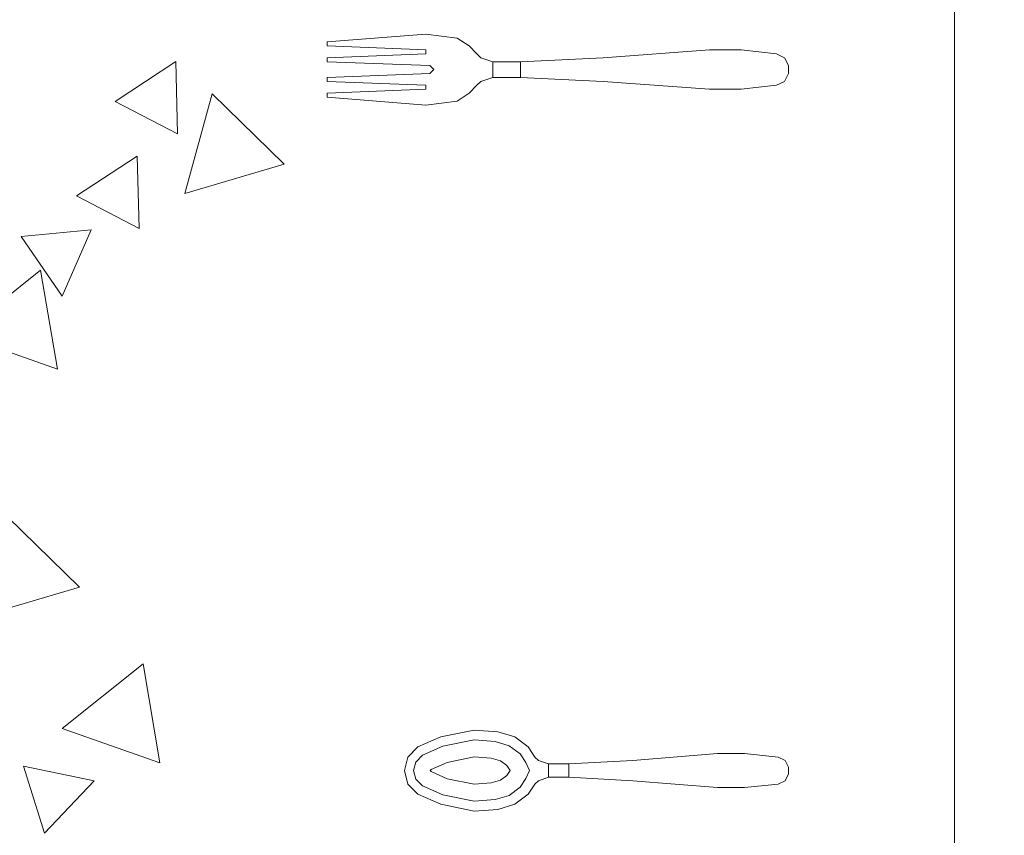
# Model space of a CAD drawing. Units: inches. Extents: x 375 to 1122, y 27 to 1069.
# Tile 37 of 155: x 731.65 to 747.02, y 283.8 to 296.54. Entities that reach past the tile are written whole.
import ezdxf

# ---------------------------------------------------------------- set-up
doc = ezdxf.new("R2010")
doc.units = ezdxf.units.IN
doc.layers.add('A-ANNO-DIMS', color=2, linetype='Continuous', lineweight=18)
doc.layers.add('Furniture', color=30, linetype='Continuous', lineweight=18)
doc.styles.get("Standard").update_dxf_attribs({"font": 'arial.ttf'})
doc.dimstyles.new('ISO-25', dxfattribs={"dimtxt": 12, "dimasz": 2.5, "dimexe": 1.5, "dimexo": 1.5, "dimtad": 1, "dimdec": 1, "dimlunit": 3, "dimtxsty": 'Standard', "dimblk": 'ARCHTICK', "dimcen": 2.5, "dimadec": 0, "dimazin": 0, "dimtfac": 1, "dimtdec": 1, "dimtmove": 0, "dimatfit": 3, "dimfxl": 1.5, "dimfxlon": 1, "dimarcsym": 0})

# ---------------------------------------------------------------- blocks, each defined once
blk = doc.blocks.new('A$C403C54AD')
for p, q in [((0.83575, 1.53256, -0.0006), (1.99923, 1.53256, -0.0006)), ((1.27568, 1.33837, -0.03581), (1.2726, 1.34298, -0.03534)), ((1.27568, 1.33837, -0.03888), (1.2726, 1.34298, -0.03842)), ((1.27287, 1.24271, -0.0006), (1.30033, 1.27073, -0.0006)), ((1.30033, 1.27073, -0.0006), (1.31179, 1.23198, -0.0006)), ((1.31179, 1.23198, -0.0006), (1.27287, 1.24271, -0.0006)), ((1.26024, 1.22842, -0.0006), (1.28849, 1.22914, -0.0006)), ((1.27579, 1.2048, -0.0006), (1.26024, 1.22842, -0.0006)), ((1.28849, 1.22914, -0.0006), (1.27579, 1.2048, -0.0006)), ((1.49552, 1.21567, -0.0006), (1.53418, 1.22227, -0.0006)), ((1.53418, 1.22227, -0.0006), (1.52076, 1.18416, -0.0006)), ((1.52076, 1.18416, -0.0006), (1.49552, 1.21567, -0.0006)), ((1.29718, 1.21338, -0.0006), (1.32543, 1.2141, -0.0006)), ((1.31273, 1.18976, -0.0006), (1.29718, 1.21338, -0.0006)), ((1.32543, 1.2141, -0.0006), (1.31273, 1.18976, -0.0006)), ((1.53546, 1.16895, -0.0006), (1.54117, 1.19665, -0.0006)), ((1.54117, 1.19665, -0.0006), (1.56166, 1.17718, -0.0006)), ((1.32856, 1.16813, -0.0006), (1.32599, 1.19547, -0.0006)), ((1.32599, 1.19547, -0.0006), (1.35188, 1.18409, -0.0006)), ((1.43807, 1.16281, -0.0006), (1.46553, 1.19082, -0.0006)), ((1.46553, 1.19082, -0.0006), (1.47699, 1.15208, -0.0006)), ((1.35188, 1.18409, -0.0006), (1.32856, 1.16813, -0.0006)), ((1.34169, 1.17565, -0.0006), (1.38035, 1.18225, -0.0006)), ((1.38035, 1.18225, -0.0006), (1.36693, 1.14415, -0.0006)), ((1.56166, 1.17718, -0.0006), (1.53546, 1.16895, -0.0006)), ((1.36693, 1.14415, -0.0006), (1.34169, 1.17565, -0.0006))]:
    blk.add_line(p, q)
for points, invisible_edges in [([(1.25875, 1.46612, -0.03397), (1.26799, 1.46612, -0.03397), (1.26953, 1.46304, -0.03421), (1.25721, 1.46304, -0.03421)], 5), ([(1.25875, 1.46612, -0.0386), (1.26799, 1.46612, -0.0386), (1.26953, 1.46304, -0.03884), (1.25721, 1.46304, -0.03884)], 5), ([(1.26491, 1.46766, -0.03413), (1.26183, 1.46766, -0.03413), (1.25875, 1.46612, -0.03397), (1.26799, 1.46612, -0.03397)], 4), ([(1.26491, 1.46766, -0.03827), (1.26183, 1.46766, -0.03827), (1.25875, 1.46612, -0.0386), (1.26799, 1.46612, -0.0386)], 4), ([(1.53323, 1.46634, -0.04237), (1.54115, 1.46634, -0.04237), (1.54247, 1.4637, -0.04257), (1.53191, 1.4637, -0.04257)], 5), ([(1.53323, 1.46634, -0.04634), (1.54115, 1.46634, -0.04634), (1.54247, 1.4637, -0.04655), (1.53191, 1.4637, -0.04655)], 5), ([(1.53851, 1.46766, -0.04251), (1.53587, 1.46766, -0.04251), (1.53323, 1.46634, -0.04237), (1.54115, 1.46634, -0.04237)], 4), ([(1.53851, 1.46766, -0.04605), (1.53587, 1.46766, -0.04605), (1.53323, 1.46634, -0.04634), (1.54115, 1.46634, -0.04634)], 4), ([(1.26953, 1.46304, -0.03421), (1.25721, 1.46304, -0.03421), (1.25567, 1.44919, -0.03425), (1.27106, 1.44919, -0.03425)], 5), ([(1.26953, 1.46304, -0.03884), (1.25721, 1.46304, -0.03884), (1.25567, 1.44919, -0.03888), (1.27106, 1.44919, -0.03888)], 5), ([(1.54247, 1.4637, -0.04257), (1.53191, 1.4637, -0.04257), (1.53059, 1.45051, -0.0426), (1.54379, 1.45051, -0.0426)], 5), ([(1.54247, 1.4637, -0.04655), (1.53191, 1.4637, -0.04655), (1.53059, 1.45051, -0.04658), (1.54379, 1.45051, -0.04658)], 5), ([(1.53059, 1.45051, -0.0426), (1.54379, 1.45051, -0.0426), (1.54379, 1.43995, -0.04232), (1.53059, 1.43995, -0.04232)], 5), ([(1.53059, 1.45051, -0.04658), (1.54379, 1.45051, -0.04658), (1.54379, 1.43995, -0.0463), (1.53059, 1.43995, -0.0463)], 5), ([(1.25567, 1.44919, -0.03425), (1.27106, 1.44919, -0.03425), (1.27106, 1.43687, -0.03392), (1.25567, 1.43687, -0.03392)], 5), ([(1.25567, 1.44919, -0.03888), (1.27106, 1.44919, -0.03888), (1.27106, 1.43687, -0.03855), (1.25567, 1.43687, -0.03855)], 5), ([(1.54379, 1.43995, -0.0463), (1.53059, 1.43995, -0.0463), (1.53323, 1.40697, -0.04292), (1.54115, 1.40697, -0.04292)], 5), ([(1.53059, 1.43995, -0.0463), (1.53059, 1.43995, -0.04232), (1.53323, 1.40697, -0.04028), (1.53323, 1.40697, -0.04292)], 4), ([(1.54379, 1.43995, -0.04232), (1.53059, 1.43995, -0.04232), (1.53323, 1.40697, -0.04028), (1.54115, 1.40697, -0.04028)], 5), ([(1.54115, 1.40697, -0.04292), (1.54115, 1.40697, -0.04028), (1.54379, 1.43995, -0.04232), (1.54379, 1.43995, -0.0463)], 1), ([(1.27106, 1.43687, -0.03392), (1.25567, 1.43687, -0.03392), (1.25875, 1.39532, -0.03153), (1.26799, 1.39532, -0.03153)], 5), ([(1.27106, 1.43687, -0.03855), (1.25567, 1.43687, -0.03855), (1.25875, 1.39532, -0.03461), (1.26799, 1.39532, -0.03461)], 5), ([(1.25567, 1.43687, -0.03855), (1.25567, 1.43687, -0.03392), (1.25875, 1.39532, -0.03153), (1.25875, 1.39532, -0.03461)], 4), ([(1.26799, 1.39532, -0.03461), (1.26799, 1.39532, -0.03153), (1.27106, 1.43687, -0.03392), (1.27106, 1.43687, -0.03855)], 1), ([(1.53323, 1.40697, -0.04028), (1.54115, 1.40697, -0.04028), (1.53983, 1.3819, -0.03779), (1.53455, 1.3819, -0.03779)], 1), ([(1.53323, 1.40697, -0.04028), (1.53323, 1.40697, -0.04292), (1.53455, 1.3819, -0.04001), (1.53455, 1.3819, -0.03779)], 5), ([(1.53323, 1.40697, -0.04292), (1.54115, 1.40697, -0.04292), (1.53983, 1.3819, -0.04001), (1.53455, 1.3819, -0.04001)], 1), ([(1.53983, 1.3819, -0.03779), (1.53983, 1.3819, -0.04001), (1.54115, 1.40697, -0.04292), (1.54115, 1.40697, -0.04028)], 5), ([(1.25875, 1.39532, -0.03153), (1.26799, 1.39532, -0.03153), (1.26645, 1.36299, -0.02863), (1.26029, 1.36299, -0.02863)], 1), ([(1.25875, 1.39532, -0.03153), (1.25875, 1.39532, -0.03461), (1.26029, 1.36299, -0.03122), (1.26029, 1.36299, -0.02863)], 5), ([(1.25875, 1.39532, -0.03461), (1.26799, 1.39532, -0.03461), (1.26645, 1.36299, -0.03122), (1.26029, 1.36299, -0.03122)], 1), ([(1.26645, 1.36299, -0.02863), (1.26645, 1.36299, -0.03122), (1.26799, 1.39532, -0.03461), (1.26799, 1.39532, -0.03153)], 5), ([(1.53455, 1.3819, -0.04001), (1.53455, 1.3819, -0.03779), (1.53455, 1.37399, -0.03842), (1.53455, 1.37399, -0.04064)], 5), ([(1.53983, 1.37399, -0.04064), (1.53983, 1.37399, -0.03842), (1.53983, 1.3819, -0.03779), (1.53983, 1.3819, -0.04001)], 5), ([(1.53455, 1.37399, -0.03842), (1.53983, 1.37399, -0.03842), (1.54115, 1.37003, -0.04027), (1.53323, 1.37003, -0.04027)], 4), ([(1.53455, 1.37399, -0.03842), (1.53455, 1.37399, -0.04064), (1.53323, 1.37003, -0.04236), (1.53323, 1.37003, -0.04027)], 5), ([(1.53455, 1.37399, -0.04064), (1.53983, 1.37399, -0.04064), (1.54115, 1.37003, -0.04236), (1.53323, 1.37003, -0.04236)], 4), ([(1.53983, 1.37399, -0.04064), (1.53983, 1.37399, -0.03842), (1.54115, 1.37003, -0.04027), (1.54115, 1.37003, -0.04236)], 5), ([(1.53405, 1.36518, -0.04424), (1.53191, 1.3687, -0.04315), (1.52796, 1.36608, -0.04195), (1.53064, 1.36289, -0.04423)], 5), ([(1.53405, 1.36518, -0.04292), (1.53191, 1.3687, -0.041), (1.52796, 1.36608, -0.04063), (1.53064, 1.36289, -0.04291)], 5), ([(1.54115, 1.37003, -0.04027), (1.53323, 1.37003, -0.04027), (1.53191, 1.3687, -0.041), (1.54247, 1.3687, -0.041)], 5), ([(1.54115, 1.37003, -0.04236), (1.53323, 1.37003, -0.04236), (1.53191, 1.3687, -0.04315), (1.54247, 1.3687, -0.04315)], 5), ([(1.53323, 1.37003, -0.04236), (1.53323, 1.37003, -0.04027), (1.53191, 1.3687, -0.041), (1.53191, 1.3687, -0.04315)], 1), ([(1.53191, 1.3687, -0.04315), (1.53719, 1.3687, -0.04315), (1.53719, 1.36654, -0.04406), (1.53405, 1.36518, -0.04424)], 11), ([(1.53191, 1.3687, -0.041), (1.53719, 1.3687, -0.041), (1.53719, 1.36654, -0.04274), (1.53405, 1.36518, -0.04292)], 11), ([(1.54247, 1.3687, -0.04315), (1.53719, 1.3687, -0.04315), (1.53719, 1.36654, -0.04406), (1.54033, 1.36518, -0.04424)], 11), ([(1.54247, 1.3687, -0.041), (1.53719, 1.3687, -0.041), (1.53719, 1.36654, -0.04274), (1.54033, 1.36518, -0.04292)], 11), ([(1.54033, 1.36518, -0.04292), (1.54247, 1.3687, -0.041), (1.54643, 1.36608, -0.04063), (1.54374, 1.36289, -0.04291)], 5), ([(1.54115, 1.37003, -0.04027), (1.54115, 1.37003, -0.04236), (1.54247, 1.3687, -0.04315), (1.54247, 1.3687, -0.041)], 1), ([(1.52796, 1.36608, -0.04195), (1.53064, 1.36289, -0.04423), (1.52749, 1.35867, -0.04406), (1.524, 1.36082, -0.04147)], 5), ([(1.52796, 1.36608, -0.04063), (1.53064, 1.36289, -0.04291), (1.52749, 1.35867, -0.04274), (1.524, 1.36082, -0.04015)], 5), ([(1.53523, 1.35767, -0.04647), (1.53064, 1.36289, -0.04423), (1.53405, 1.36518, -0.04424), (1.53719, 1.35902, -0.04627)], 5), ([(1.53523, 1.35767, -0.04515), (1.53064, 1.36289, -0.04291), (1.53405, 1.36518, -0.04292), (1.53719, 1.35902, -0.04495)], 5), ([(1.53405, 1.36518, -0.04424), (1.53719, 1.35902, -0.04627), (1.53719, 1.35902, -0.04627), (1.53719, 1.36654, -0.04406)], 5), ([(1.53405, 1.36518, -0.04292), (1.53719, 1.35902, -0.04495), (1.53719, 1.35902, -0.04495), (1.53719, 1.36654, -0.04274)], 5), ([(1.54033, 1.36518, -0.04424), (1.53719, 1.35902, -0.04627), (1.53719, 1.35902, -0.04627), (1.53719, 1.36654, -0.04406)], 5), ([(1.54033, 1.36518, -0.04292), (1.53719, 1.35902, -0.04495), (1.53719, 1.35902, -0.04495), (1.53719, 1.36654, -0.04274)], 5), ([(1.53915, 1.35767, -0.04647), (1.54374, 1.36289, -0.04423), (1.54033, 1.36518, -0.04424), (1.53719, 1.35902, -0.04627)], 5), ([(1.53915, 1.35767, -0.04515), (1.54374, 1.36289, -0.04291), (1.54033, 1.36518, -0.04292), (1.53719, 1.35902, -0.04495)], 5), ([(1.54643, 1.36608, -0.04195), (1.54374, 1.36289, -0.04423), (1.54689, 1.35867, -0.04406), (1.55038, 1.36082, -0.04147)], 5), ([(1.54643, 1.36608, -0.04063), (1.54374, 1.36289, -0.04291), (1.54689, 1.35867, -0.04274), (1.55038, 1.36082, -0.04015)], 5), ([(1.26029, 1.36299, -0.03122), (1.26029, 1.36299, -0.02863), (1.26029, 1.35222, -0.03071), (1.26029, 1.35222, -0.0333)], 5), ([(1.26645, 1.35222, -0.0333), (1.26645, 1.35222, -0.03071), (1.26645, 1.36299, -0.02863), (1.26645, 1.36299, -0.03122)], 5), ([(1.52749, 1.35867, -0.04406), (1.53346, 1.3553, -0.04638), (1.53523, 1.35767, -0.04647), (1.53064, 1.36289, -0.04423)], 5), ([(1.52749, 1.35867, -0.04274), (1.53346, 1.3553, -0.04506), (1.53523, 1.35767, -0.04515), (1.53064, 1.36289, -0.04291)], 5), ([(1.54689, 1.35867, -0.04406), (1.54092, 1.3553, -0.04638), (1.53915, 1.35767, -0.04647), (1.54374, 1.36289, -0.04423)], 5), ([(1.54689, 1.35867, -0.04274), (1.54092, 1.3553, -0.04506), (1.53915, 1.35767, -0.04515), (1.54374, 1.36289, -0.04291)], 5), ([(1.52749, 1.35867, -0.04274), (1.524, 1.36082, -0.04015), (1.52202, 1.35422, -0.03974), (1.52583, 1.35316, -0.04222)], 5), ([(1.52749, 1.35867, -0.04406), (1.524, 1.36082, -0.04147), (1.52202, 1.35422, -0.04106), (1.52583, 1.35316, -0.04354)], 5), ([(1.53234, 1.35158, -0.04614), (1.52583, 1.35316, -0.04354), (1.52749, 1.35867, -0.04406), (1.53346, 1.3553, -0.04638)], 5), ([(1.53234, 1.35158, -0.04482), (1.52583, 1.35316, -0.04222), (1.52749, 1.35867, -0.04274), (1.53346, 1.3553, -0.04506)], 5), ([(1.54092, 1.3553, -0.04638), (1.53346, 1.3553, -0.04638), (1.53523, 1.35767, -0.04647), (1.53915, 1.35767, -0.04647)], 5), ([(1.54092, 1.3553, -0.04506), (1.53346, 1.3553, -0.04506), (1.53523, 1.35767, -0.04515), (1.53915, 1.35767, -0.04515)], 5), ([(1.53523, 1.35767, -0.04647), (1.53915, 1.35767, -0.04647), (1.53719, 1.35902, -0.04627)], 1), ([(1.53523, 1.35767, -0.04515), (1.53915, 1.35767, -0.04515), (1.53719, 1.35902, -0.04495)], 1), ([(1.54204, 1.35158, -0.04482), (1.54855, 1.35316, -0.04222), (1.54689, 1.35867, -0.04274), (1.54092, 1.3553, -0.04506)], 5), ([(1.54689, 1.35867, -0.04274), (1.55038, 1.36082, -0.04015), (1.55236, 1.35422, -0.03974), (1.54855, 1.35316, -0.04222)], 5), ([(1.54689, 1.35867, -0.04406), (1.55038, 1.36082, -0.04147), (1.55236, 1.35422, -0.04106), (1.54855, 1.35316, -0.04354)], 5), ([(1.52202, 1.35422, -0.03974), (1.52583, 1.35316, -0.04222), (1.52524, 1.34491, -0.04133), (1.52136, 1.34501, -0.03888)], 5), ([(1.52202, 1.35422, -0.04106), (1.52583, 1.35316, -0.04354), (1.52524, 1.34491, -0.04265), (1.52136, 1.34501, -0.0402)], 5), ([(1.53234, 1.35158, -0.04614), (1.54204, 1.35158, -0.04614), (1.54092, 1.3553, -0.04638), (1.53346, 1.3553, -0.04638)], 5), ([(1.53234, 1.35158, -0.04482), (1.54204, 1.35158, -0.04482), (1.54092, 1.3553, -0.04506), (1.53346, 1.3553, -0.04506)], 5), ([(1.55236, 1.35422, -0.03974), (1.54855, 1.35316, -0.04222), (1.54914, 1.34491, -0.04133), (1.55302, 1.34501, -0.03888)], 5), ([(1.55236, 1.35422, -0.04106), (1.54855, 1.35316, -0.04354), (1.54914, 1.34491, -0.04265), (1.55302, 1.34501, -0.0402)], 5), ([(1.26029, 1.35222, -0.03071), (1.26645, 1.35222, -0.03071), (1.26799, 1.3476, -0.03306), (1.25875, 1.3476, -0.03306)], 4), ([(1.26029, 1.35222, -0.0333), (1.26645, 1.35222, -0.0333), (1.26799, 1.3476, -0.03584), (1.25875, 1.3476, -0.03584)], 4), ([(1.26029, 1.35222, -0.03071), (1.26029, 1.35222, -0.0333), (1.25875, 1.3476, -0.03584), (1.25875, 1.3476, -0.03306)], 5), ([(1.26645, 1.35222, -0.0333), (1.26645, 1.35222, -0.03071), (1.26799, 1.3476, -0.03306), (1.26799, 1.3476, -0.03584)], 5), ([(1.52524, 1.34491, -0.04265), (1.53187, 1.34497, -0.0452), (1.53234, 1.35158, -0.04614), (1.52583, 1.35316, -0.04354)], 5), ([(1.52524, 1.34491, -0.04133), (1.53187, 1.34497, -0.04388), (1.53234, 1.35158, -0.04482), (1.52583, 1.35316, -0.04222)], 5), ([(1.54252, 1.34497, -0.0452), (1.53187, 1.34497, -0.0452), (1.53234, 1.35158, -0.04614), (1.54204, 1.35158, -0.04614)], 5), ([(1.54252, 1.34497, -0.04388), (1.53187, 1.34497, -0.04388), (1.53234, 1.35158, -0.04482), (1.54204, 1.35158, -0.04482)], 5), ([(1.54914, 1.34491, -0.04265), (1.54252, 1.34497, -0.0452), (1.54204, 1.35158, -0.04614), (1.54855, 1.35316, -0.04354)], 5), ([(1.54914, 1.34491, -0.04133), (1.54252, 1.34497, -0.04388), (1.54204, 1.35158, -0.04482), (1.54855, 1.35316, -0.04222)], 5), ([(1.26953, 1.34606, -0.03718), (1.25721, 1.34606, -0.03718), (1.25413, 1.34298, -0.03842), (1.2726, 1.34298, -0.03842)], 5), ([(1.26953, 1.34606, -0.0341), (1.25721, 1.34606, -0.0341), (1.25413, 1.34298, -0.03534), (1.2726, 1.34298, -0.03534)], 5), ([(1.26799, 1.3476, -0.03306), (1.25875, 1.3476, -0.03306), (1.25721, 1.34606, -0.0341), (1.26953, 1.34606, -0.0341)], 5), ([(1.26799, 1.3476, -0.03584), (1.25875, 1.3476, -0.03584), (1.25721, 1.34606, -0.03718), (1.26953, 1.34606, -0.03718)], 5), ([(1.25875, 1.3476, -0.03584), (1.25875, 1.3476, -0.03306), (1.25721, 1.34606, -0.0341), (1.25721, 1.34606, -0.03718)], 1), ([(1.26799, 1.3476, -0.03306), (1.26799, 1.3476, -0.03584), (1.26953, 1.34606, -0.03718), (1.26953, 1.34606, -0.0341)], 1), ([(1.25413, 1.34298, -0.03534), (1.2726, 1.34298, -0.03534), (1.27568, 1.33837, -0.03581), (1.25105, 1.33837, -0.03581)], 5), ([(1.25413, 1.34298, -0.03842), (1.2726, 1.34298, -0.03842), (1.27568, 1.33837, -0.03888), (1.25105, 1.33837, -0.03888)], 5), ([(1.25413, 1.34298, -0.03842), (1.25413, 1.34298, -0.03534), (1.25105, 1.33837, -0.03581), (1.25105, 1.33837, -0.03888)], 4), ([(1.2726, 1.34298, -0.03534), (1.2726, 1.34298, -0.03842), (1.27568, 1.33837, -0.03888), (1.27568, 1.33837, -0.03581)], 4), ([(1.52524, 1.34491, -0.04265), (1.52136, 1.34501, -0.0402), (1.524, 1.33198, -0.03816), (1.5277, 1.33278, -0.04067)], 5), ([(1.52524, 1.34491, -0.04133), (1.52136, 1.34501, -0.03888), (1.524, 1.33198, -0.03684), (1.5277, 1.33278, -0.03935)], 5), ([(1.53402, 1.33436, -0.04216), (1.5277, 1.33278, -0.03935), (1.52524, 1.34491, -0.04133), (1.53187, 1.34497, -0.04388)], 5), ([(1.53402, 1.33436, -0.04348), (1.5277, 1.33278, -0.04067), (1.52524, 1.34491, -0.04265), (1.53187, 1.34497, -0.0452)], 5), ([(1.53402, 1.33436, -0.04216), (1.54037, 1.33436, -0.04216), (1.54252, 1.34497, -0.04388), (1.53187, 1.34497, -0.04388)], 5), ([(1.53402, 1.33436, -0.04348), (1.54037, 1.33436, -0.04348), (1.54252, 1.34497, -0.0452), (1.53187, 1.34497, -0.0452)], 5), ([(1.54037, 1.33436, -0.04216), (1.54668, 1.33278, -0.03935), (1.54914, 1.34491, -0.04133), (1.54252, 1.34497, -0.04388)], 5), ([(1.54037, 1.33436, -0.04348), (1.54668, 1.33278, -0.04067), (1.54914, 1.34491, -0.04265), (1.54252, 1.34497, -0.0452)], 5), ([(1.54914, 1.34491, -0.04265), (1.55302, 1.34501, -0.0402), (1.55038, 1.33198, -0.03816), (1.54668, 1.33278, -0.04067)], 5), ([(1.54914, 1.34491, -0.04133), (1.55302, 1.34501, -0.03888), (1.55038, 1.33198, -0.03684), (1.54668, 1.33278, -0.03935)], 5), ([(1.25105, 1.33837, -0.03581), (1.25721, 1.32605, -0.03521), (1.25567, 1.32605, -0.03521), (1.24952, 1.32605, -0.03521)], 5), ([(1.25105, 1.33837, -0.03888), (1.25721, 1.32605, -0.03829), (1.25567, 1.32605, -0.03829), (1.24952, 1.32605, -0.03829)], 5), ([(1.25105, 1.33837, -0.03581), (1.25105, 1.33837, -0.03888), (1.24952, 1.32605, -0.03829), (1.24952, 1.32605, -0.03521)], 1), ([(1.25105, 1.33837, -0.03581), (1.26337, 1.32925, -0.0356), (1.26183, 1.32759, -0.03545), (1.25721, 1.32605, -0.03521)], 13), ([(1.25105, 1.33837, -0.03581), (1.26337, 1.32925, -0.0356), (1.27568, 1.33837, -0.03581), (1.25105, 1.33837, -0.03581)], 7), ([(1.25105, 1.33837, -0.03888), (1.26337, 1.32925, -0.03868), (1.26183, 1.32759, -0.03853), (1.25721, 1.32605, -0.03829)], 13), ([(1.25105, 1.33837, -0.03888), (1.26337, 1.32925, -0.03868), (1.27568, 1.33837, -0.03888), (1.25105, 1.33837, -0.03888)], 7), ([(1.27568, 1.33837, -0.03581), (1.26337, 1.32925, -0.0356), (1.26491, 1.32759, -0.03545), (1.26953, 1.32605, -0.03521)], 13), ([(1.27568, 1.33837, -0.03888), (1.26337, 1.32925, -0.03868), (1.26491, 1.32759, -0.03853), (1.26953, 1.32605, -0.03829)], 13), ([(1.27568, 1.33837, -0.03581), (1.26953, 1.32605, -0.03521), (1.27106, 1.32605, -0.03521), (1.27722, 1.32605, -0.03521)], 5), ([(1.27568, 1.33837, -0.03888), (1.26953, 1.32605, -0.03829), (1.27106, 1.32605, -0.03829), (1.27722, 1.32605, -0.03829)], 5), ([(1.27568, 1.33837, -0.03888), (1.27568, 1.33837, -0.03581), (1.27722, 1.32605, -0.03521), (1.27722, 1.32605, -0.03829)], 1), ([(1.53121, 1.32476, -0.03896), (1.53675, 1.32814, -0.04186), (1.53402, 1.33436, -0.04348), (1.5277, 1.33278, -0.04067)], 5), ([(1.53121, 1.32476, -0.03764), (1.53675, 1.32814, -0.04054), (1.53402, 1.33436, -0.04216), (1.5277, 1.33278, -0.03935)], 5), ([(1.53763, 1.32814, -0.04186), (1.53675, 1.32814, -0.04186), (1.53402, 1.33436, -0.04348), (1.54037, 1.33436, -0.04348)], 5), ([(1.53763, 1.32814, -0.04054), (1.53675, 1.32814, -0.04054), (1.53402, 1.33436, -0.04216), (1.54037, 1.33436, -0.04216)], 5), ([(1.54318, 1.32476, -0.03896), (1.53763, 1.32814, -0.04186), (1.54037, 1.33436, -0.04348), (1.54668, 1.33278, -0.04067)], 5), ([(1.54318, 1.32476, -0.03764), (1.53763, 1.32814, -0.04054), (1.54037, 1.33436, -0.04216), (1.54668, 1.33278, -0.03935)], 5), ([(1.524, 1.33198, -0.03816), (1.5277, 1.33278, -0.04067), (1.53121, 1.32476, -0.03896), (1.52796, 1.32291, -0.03632)], 5), ([(1.524, 1.33198, -0.03684), (1.5277, 1.33278, -0.03935), (1.53121, 1.32476, -0.03764), (1.52796, 1.32291, -0.035)], 5), ([(1.55038, 1.33198, -0.03816), (1.54668, 1.33278, -0.04067), (1.54318, 1.32476, -0.03896), (1.54643, 1.32291, -0.03632)], 5), ([(1.55038, 1.33198, -0.03684), (1.54668, 1.33278, -0.03935), (1.54318, 1.32476, -0.03764), (1.54643, 1.32291, -0.035)], 5), ([(1.25721, 1.32605, -0.03521), (1.26183, 1.32759, -0.03545), (1.26029, 1.28757, -0.02811), (1.25875, 1.28757, -0.02811)], 1), ([(1.25721, 1.32605, -0.03829), (1.26183, 1.32759, -0.03853), (1.26029, 1.28757, -0.03119), (1.25875, 1.28757, -0.03119)], 1), ([(1.26491, 1.32759, -0.03545), (1.26953, 1.32605, -0.03521), (1.26799, 1.28757, -0.02811), (1.26645, 1.28757, -0.02811)], 1), ([(1.26491, 1.32759, -0.03853), (1.26953, 1.32605, -0.03829), (1.26799, 1.28757, -0.03119), (1.26645, 1.28757, -0.03119)], 1), ([(1.53675, 1.32814, -0.04054), (1.53388, 1.32213, -0.03709), (1.53121, 1.32476, -0.03764), (1.53675, 1.32814, -0.04054)], 5), ([(1.53675, 1.32814, -0.04186), (1.53388, 1.32213, -0.03841), (1.53121, 1.32476, -0.03896), (1.53675, 1.32814, -0.04186)], 5), ([(1.53719, 1.32132, -0.0369), (1.53719, 1.32772, -0.0404), (1.53675, 1.32814, -0.04054), (1.53388, 1.32213, -0.03709)], 5), ([(1.53719, 1.32132, -0.03822), (1.53719, 1.32772, -0.04172), (1.53675, 1.32814, -0.04186), (1.53388, 1.32213, -0.03841)], 5), ([(1.53719, 1.32772, -0.0404), (1.53675, 1.32814, -0.04054), (1.53763, 1.32814, -0.04054), (1.53719, 1.32772, -0.0404)], 2), ([(1.53719, 1.32772, -0.04172), (1.53675, 1.32814, -0.04186), (1.53763, 1.32814, -0.04186), (1.53719, 1.32772, -0.04172)], 2), ([(1.53719, 1.32132, -0.0369), (1.53719, 1.32772, -0.0404), (1.53763, 1.32814, -0.04054), (1.5405, 1.32213, -0.03709)], 5), ([(1.53719, 1.32132, -0.03822), (1.53719, 1.32772, -0.04172), (1.53763, 1.32814, -0.04186), (1.5405, 1.32213, -0.03841)], 5), ([(1.53763, 1.32814, -0.04054), (1.5405, 1.32213, -0.03709), (1.54318, 1.32476, -0.03764), (1.53763, 1.32814, -0.04054)], 5), ([(1.53763, 1.32814, -0.04186), (1.5405, 1.32213, -0.03841), (1.54318, 1.32476, -0.03896), (1.53763, 1.32814, -0.04186)], 5), ([(1.25567, 1.32605, -0.03521), (1.24952, 1.32605, -0.03521), (1.25259, 1.28757, -0.02811), (1.25413, 1.28757, -0.02811)], 1), ([(1.25567, 1.32605, -0.03829), (1.24952, 1.32605, -0.03829), (1.25259, 1.28757, -0.03119), (1.25413, 1.28757, -0.03119)], 1), ([(1.27106, 1.32605, -0.03521), (1.27722, 1.32605, -0.03521), (1.27414, 1.28757, -0.02811), (1.2726, 1.28757, -0.02811)], 1), ([(1.27106, 1.32605, -0.03829), (1.27722, 1.32605, -0.03829), (1.27414, 1.28757, -0.03119), (1.2726, 1.28757, -0.03119)], 1), ([(1.53121, 1.32476, -0.03896), (1.52796, 1.32291, -0.03632), (1.53191, 1.31907, -0.03523), (1.53388, 1.32213, -0.03841)], 5), ([(1.53121, 1.32476, -0.03764), (1.52796, 1.32291, -0.035), (1.53191, 1.31907, -0.03391), (1.53388, 1.32213, -0.03709)], 5), ([(1.54318, 1.32476, -0.03896), (1.54643, 1.32291, -0.03632), (1.54247, 1.31907, -0.03523), (1.5405, 1.32213, -0.03841)], 5), ([(1.54318, 1.32476, -0.03764), (1.54643, 1.32291, -0.035), (1.54247, 1.31907, -0.03391), (1.5405, 1.32213, -0.03709)], 5), ([(1.53191, 1.31907, -0.03523), (1.53388, 1.32213, -0.03841), (1.53719, 1.32132, -0.03822), (1.53719, 1.31776, -0.03505)], 5), ([(1.53191, 1.31907, -0.03391), (1.53388, 1.32213, -0.03709), (1.53719, 1.32132, -0.0369), (1.53719, 1.31776, -0.03373)], 5), ([(1.54247, 1.31907, -0.03523), (1.5405, 1.32213, -0.03841), (1.53719, 1.32132, -0.03822), (1.53719, 1.31776, -0.03505)], 5), ([(1.54247, 1.31907, -0.03391), (1.5405, 1.32213, -0.03709), (1.53719, 1.32132, -0.0369), (1.53719, 1.31776, -0.03373)], 5)]:
    blk.add_3dface(points, dxfattribs=dict(invisible_edges=invisible_edges))
for points in [[(1.25875, 1.46612, -0.03397), (1.25875, 1.46612, -0.0386), (1.25721, 1.46304, -0.03884), (1.25721, 1.46304, -0.03421)], [(1.26183, 1.46766, -0.03827), (1.26183, 1.46766, -0.03413), (1.25875, 1.46612, -0.03397), (1.25875, 1.46612, -0.0386)], [(1.26491, 1.46766, -0.03413), (1.26491, 1.46766, -0.03827), (1.26183, 1.46766, -0.03827), (1.26183, 1.46766, -0.03413)], [(1.26799, 1.46612, -0.0386), (1.26799, 1.46612, -0.03397), (1.26491, 1.46766, -0.03413), (1.26491, 1.46766, -0.03827)], [(1.26953, 1.46304, -0.03421), (1.26953, 1.46304, -0.03884), (1.26799, 1.46612, -0.0386), (1.26799, 1.46612, -0.03397)], [(1.53323, 1.46634, -0.04237), (1.53323, 1.46634, -0.04634), (1.53191, 1.4637, -0.04655), (1.53191, 1.4637, -0.04257)], [(1.53587, 1.46766, -0.04605), (1.53587, 1.46766, -0.04251), (1.53323, 1.46634, -0.04237), (1.53323, 1.46634, -0.04634)], [(1.53851, 1.46766, -0.04251), (1.53851, 1.46766, -0.04605), (1.53587, 1.46766, -0.04605), (1.53587, 1.46766, -0.04251)], [(1.54115, 1.46634, -0.04634), (1.54115, 1.46634, -0.04237), (1.53851, 1.46766, -0.04251), (1.53851, 1.46766, -0.04605)], [(1.54247, 1.4637, -0.04257), (1.54247, 1.4637, -0.04655), (1.54115, 1.46634, -0.04634), (1.54115, 1.46634, -0.04237)], [(1.25721, 1.46304, -0.03884), (1.25721, 1.46304, -0.03421), (1.25567, 1.44919, -0.03425), (1.25567, 1.44919, -0.03888)], [(1.27106, 1.44919, -0.03888), (1.27106, 1.44919, -0.03425), (1.26953, 1.46304, -0.03421), (1.26953, 1.46304, -0.03884)], [(1.53191, 1.4637, -0.04655), (1.53191, 1.4637, -0.04257), (1.53059, 1.45051, -0.0426), (1.53059, 1.45051, -0.04658)], [(1.54379, 1.45051, -0.04658), (1.54379, 1.45051, -0.0426), (1.54247, 1.4637, -0.04257), (1.54247, 1.4637, -0.04655)], [(1.53059, 1.45051, -0.0426), (1.53059, 1.45051, -0.04658), (1.53059, 1.43995, -0.0463), (1.53059, 1.43995, -0.04232)], [(1.54379, 1.43995, -0.04232), (1.54379, 1.43995, -0.0463), (1.54379, 1.45051, -0.04658), (1.54379, 1.45051, -0.0426)], [(1.25567, 1.44919, -0.03425), (1.25567, 1.44919, -0.03888), (1.25567, 1.43687, -0.03855), (1.25567, 1.43687, -0.03392)], [(1.27106, 1.43687, -0.03392), (1.27106, 1.43687, -0.03855), (1.27106, 1.44919, -0.03888), (1.27106, 1.44919, -0.03425)], [(1.53983, 1.3819, -0.04001), (1.53455, 1.3819, -0.04001), (1.53455, 1.37399, -0.04064), (1.53983, 1.37399, -0.04064)], [(1.53983, 1.3819, -0.03779), (1.53455, 1.3819, -0.03779), (1.53455, 1.37399, -0.03842), (1.53983, 1.37399, -0.03842)], [(1.53191, 1.3687, -0.04315), (1.53191, 1.3687, -0.041), (1.52796, 1.36608, -0.04063), (1.52796, 1.36608, -0.04195)], [(1.54643, 1.36608, -0.04195), (1.54643, 1.36608, -0.04063), (1.54247, 1.3687, -0.041), (1.54247, 1.3687, -0.04315)], [(1.52796, 1.36608, -0.04063), (1.52796, 1.36608, -0.04195), (1.524, 1.36082, -0.04147), (1.524, 1.36082, -0.04015)], [(1.55038, 1.36082, -0.04015), (1.55038, 1.36082, -0.04147), (1.54643, 1.36608, -0.04195), (1.54643, 1.36608, -0.04063)], [(1.26645, 1.36299, -0.02863), (1.26029, 1.36299, -0.02863), (1.26029, 1.35222, -0.03071), (1.26645, 1.35222, -0.03071)], [(1.26645, 1.36299, -0.03122), (1.26029, 1.36299, -0.03122), (1.26029, 1.35222, -0.0333), (1.26645, 1.35222, -0.0333)], [(1.524, 1.36082, -0.04147), (1.524, 1.36082, -0.04015), (1.52202, 1.35422, -0.03974), (1.52202, 1.35422, -0.04106)], [(1.55236, 1.35422, -0.04106), (1.55236, 1.35422, -0.03974), (1.55038, 1.36082, -0.04015), (1.55038, 1.36082, -0.04147)], [(1.52202, 1.35422, -0.03974), (1.52202, 1.35422, -0.04106), (1.52136, 1.34501, -0.0402), (1.52136, 1.34501, -0.03888)], [(1.55302, 1.34501, -0.0402), (1.55302, 1.34501, -0.03888), (1.55236, 1.35422, -0.03974), (1.55236, 1.35422, -0.04106)], [(1.25721, 1.34606, -0.0341), (1.25721, 1.34606, -0.03718), (1.25413, 1.34298, -0.03842), (1.25413, 1.34298, -0.03534)], [(1.26953, 1.34606, -0.03718), (1.26953, 1.34606, -0.0341), (1.2726, 1.34298, -0.03534), (1.2726, 1.34298, -0.03842)], [(1.52136, 1.34501, -0.0402), (1.52136, 1.34501, -0.03888), (1.524, 1.33198, -0.03684), (1.524, 1.33198, -0.03816)], [(1.55038, 1.33198, -0.03684), (1.55038, 1.33198, -0.03816), (1.55302, 1.34501, -0.0402), (1.55302, 1.34501, -0.03888)], [(1.524, 1.33198, -0.03684), (1.524, 1.33198, -0.03816), (1.52796, 1.32291, -0.03632), (1.52796, 1.32291, -0.035)], [(1.54643, 1.32291, -0.03632), (1.54643, 1.32291, -0.035), (1.55038, 1.33198, -0.03684), (1.55038, 1.33198, -0.03816)], [(1.26029, 1.28757, -0.03119), (1.26029, 1.28757, -0.02811), (1.26183, 1.32759, -0.03545), (1.26183, 1.32759, -0.03853)], [(1.26337, 1.32925, -0.03868), (1.26337, 1.32925, -0.0356), (1.26183, 1.32759, -0.03545), (1.26183, 1.32759, -0.03853)], [(1.26491, 1.32759, -0.03545), (1.26491, 1.32759, -0.03853), (1.26337, 1.32925, -0.03868), (1.26337, 1.32925, -0.0356)], [(1.26491, 1.32759, -0.03853), (1.26491, 1.32759, -0.03545), (1.26645, 1.28757, -0.02811), (1.26645, 1.28757, -0.03119)], [(1.24952, 1.32605, -0.03829), (1.24952, 1.32605, -0.03521), (1.25259, 1.28757, -0.02811), (1.25259, 1.28757, -0.03119)], [(1.25413, 1.28757, -0.02811), (1.25413, 1.28757, -0.03119), (1.25567, 1.32605, -0.03829), (1.25567, 1.32605, -0.03521)], [(1.25721, 1.32605, -0.03829), (1.25721, 1.32605, -0.03521), (1.25567, 1.32605, -0.03521), (1.25567, 1.32605, -0.03829)], [(1.25721, 1.32605, -0.03829), (1.25721, 1.32605, -0.03521), (1.25875, 1.28757, -0.02811), (1.25875, 1.28757, -0.03119)], [(1.26799, 1.28757, -0.02811), (1.26799, 1.28757, -0.03119), (1.26953, 1.32605, -0.03829), (1.26953, 1.32605, -0.03521)], [(1.27106, 1.32605, -0.03521), (1.27106, 1.32605, -0.03829), (1.26953, 1.32605, -0.03829), (1.26953, 1.32605, -0.03521)], [(1.27106, 1.32605, -0.03521), (1.27106, 1.32605, -0.03829), (1.2726, 1.28757, -0.03119), (1.2726, 1.28757, -0.02811)], [(1.27414, 1.28757, -0.02811), (1.27414, 1.28757, -0.03119), (1.27722, 1.32605, -0.03829), (1.27722, 1.32605, -0.03521)], [(1.52796, 1.32291, -0.03632), (1.52796, 1.32291, -0.035), (1.53191, 1.31907, -0.03391), (1.53191, 1.31907, -0.03523)], [(1.54247, 1.31907, -0.03391), (1.54247, 1.31907, -0.03523), (1.54643, 1.32291, -0.03632), (1.54643, 1.32291, -0.035)], [(1.53191, 1.31907, -0.03391), (1.53191, 1.31907, -0.03523), (1.53719, 1.31776, -0.03505), (1.53719, 1.31776, -0.03373)], [(1.53719, 1.31776, -0.03505), (1.53719, 1.31776, -0.03373), (1.54247, 1.31907, -0.03391), (1.54247, 1.31907, -0.03523)], [(1.25259, 1.28757, -0.03119), (1.25259, 1.28757, -0.02811), (1.25413, 1.28757, -0.02811), (1.25413, 1.28757, -0.03119)], [(1.25875, 1.28757, -0.03119), (1.25875, 1.28757, -0.02811), (1.26029, 1.28757, -0.02811), (1.26029, 1.28757, -0.03119)], [(1.26645, 1.28757, -0.03119), (1.26645, 1.28757, -0.02811), (1.26799, 1.28757, -0.02811), (1.26799, 1.28757, -0.03119)], [(1.2726, 1.28757, -0.03119), (1.2726, 1.28757, -0.02811), (1.27414, 1.28757, -0.02811), (1.27414, 1.28757, -0.03119)]]:
    blk.add_3dface(points)
blk = doc.blocks.new('_ArchTick')
at = {"color": 0, "linetype": 'ByBlock', "const_width": 0.15}
blk.add_lwpolyline([(-0.5, -0.5), (0.5, 0.5)], dxfattribs=at)
blk = doc.blocks.new('*D94')
at = {"layer": 'A-ANNO-DIMS', "color": 0, "lineweight": -2, "transparency": 16777216}
for p, q in [((734.007, 117.528), (734.007, 114.528)), ((773.007, 117.528), (773.007, 114.528)), ((734.007, 116.028), (773.007, 116.028))]:
    blk.add_line(p, q, dxfattribs=at)
at = {"layer": 'Defpoints', "color": 0, "transparency": 16777216}
for p in [(734.007, 667.528), (773.007, 667.528), (773.007, 116.028)]:
    blk.add_point(p, dxfattribs=at)
at = {"layer": 'A-ANNO-DIMS', "color": 0, "lineweight": -2, "transparency": 16777216, "xscale": 2.5, "yscale": 2.5, "zscale": 2.5, "rotation": 180}
blk.add_blockref('_ArchTick', (734.007, 116.028), dxfattribs=at)
at = {"layer": 'A-ANNO-DIMS', "color": 0, "lineweight": -2, "transparency": 16777216, "xscale": 2.5, "yscale": 2.5, "zscale": 2.5}
blk.add_blockref('_ArchTick', (773.007, 116.028), dxfattribs=at)
at = {"layer": 'A-ANNO-DIMS', "color": 0, "transparency": 16777216, "insert": (753.507, 122.784), "char_height": 12, "attachment_point": 5}
blk.add_mtext('3\'-3"', dxfattribs=at)

msp = doc.modelspace()

# ---------------------------------------------------------------- block references
at = {"layer": 'Furniture', "xscale": 39.9918517141215, "yscale": 39.9918517141215, "zscale": 39.9918517141215, "rotation": 270}
msp.add_blockref('A$C403C54AD', (684.955, 346.287, 0.024), dxfattribs=at)

# ---------------------------------------------------------------- dimensions: what is measured, and where the dimension line sits
at = {"layer": 'A-ANNO-DIMS'}
dim = msp.add_linear_dim(base=(773.007, 116.028), p1=(734.007, 667.528), p2=(773.007, 667.528), dimstyle='ISO-25', override={"dimdec": 1, "dimlfac": 1, "dimrnd": 0, "dimzin": 1, "dimdsep": 46, "dimlunit": 4, "dimfrac": 2}, dxfattribs=at)
dim.commit()
dim.dimension.update_dxf_attribs({"geometry": '*D94', "text_midpoint": (753.507, 122.784)})

doc.saveas('drawing.dxf')
